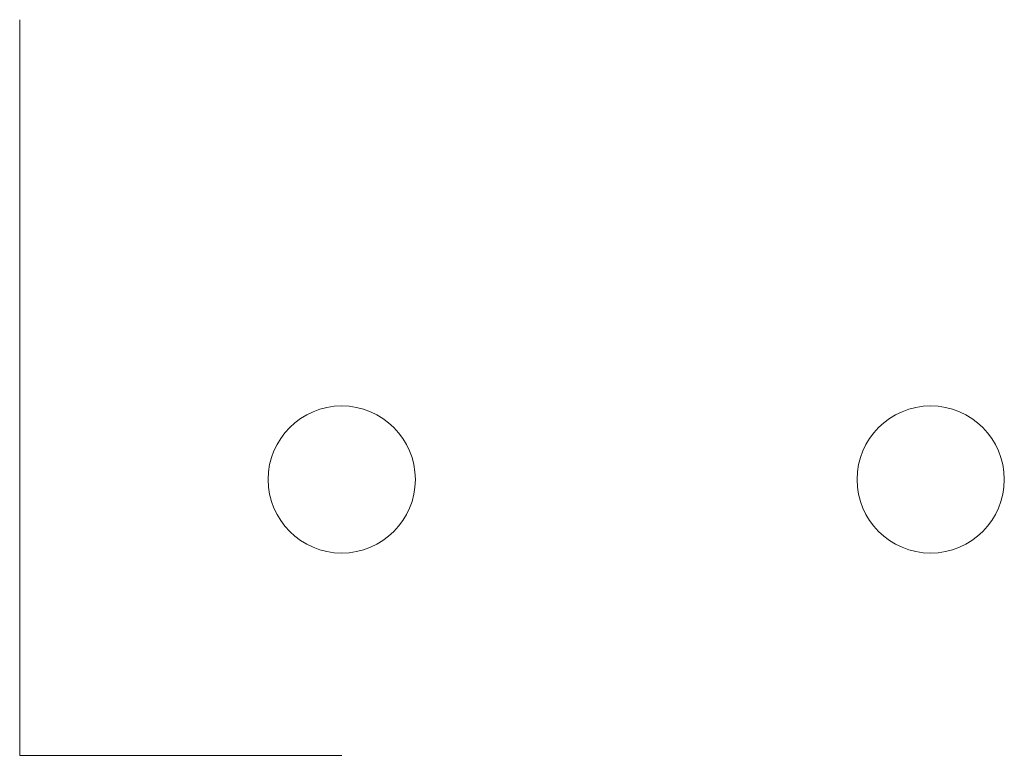
# Model space of a CAD drawing. Units: millimetres. Extents: x 3114 to 3221, y 1563 to 1643.
import ezdxf

# ---------------------------------------------------------------- set-up
doc = ezdxf.new("R2010")
doc.units = ezdxf.units.MM
doc.layers.add('M-CONS', color=8, linetype='Continuous', lineweight=13)

msp = doc.modelspace()

# ---------------------------------------------------------------- linework, layer by layer
at = {"layer": 'M-CONS'}
msp.add_line((3113.57, 1563.27, 9), (3148.57, 1563.27, 9), dxfattribs=at)
at = {"layer": 'M-CONS', "extrusion": (1, -1e-16, 1e-16), "elevation": 3113.57}
msp.add_lwpolyline([(1581.27, -6), (1581.27, -9), (1563.27, -9), (1563.27, 9), (1643.27, 9), (1643.27, -9), (1625.27, -9), (1625.27, -6)], close=True, dxfattribs=at)
at = {"layer": 'M-CONS'}
for centre in [(3148.57, 1593.27, 9), (3212.57, 1593.27, 9)]:
    msp.add_circle(centre, 8, dxfattribs=at)

doc.saveas('drawing.dxf')
